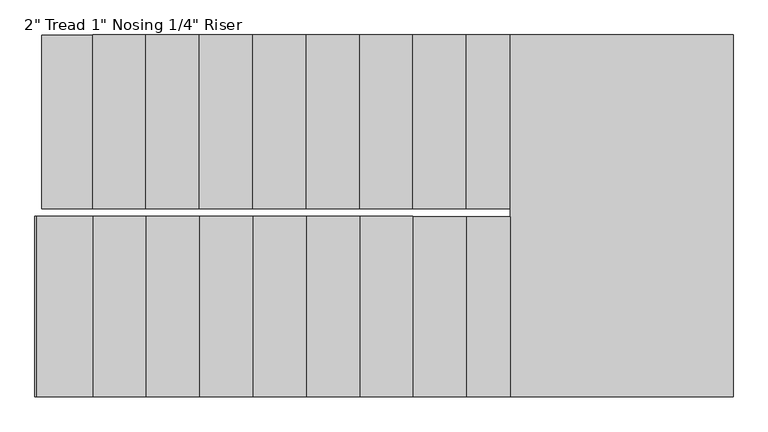
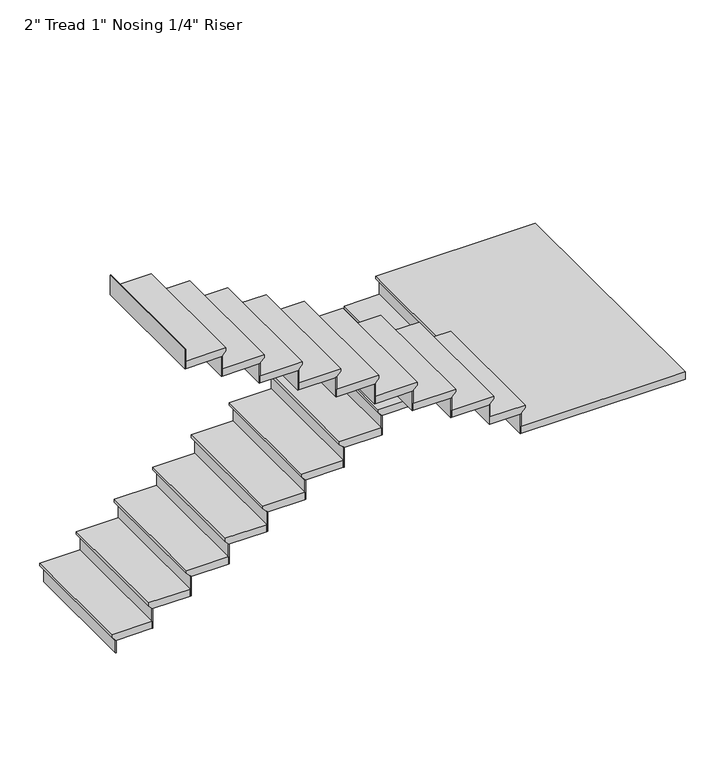
"""IFC4 building model written with IfcOpenShell, lengths in millimetres: stair flight geometry."""

from ifc_helpers import new_model, si_unit, origin, place, context, project, spatial, faceted_brep, source, transform, mapped, element, save


def stair_flight_3990532a(model_context):
    return source(origin(), model_context, "Body", "Brep", [
        faceted_brep([(1537.1941283, 180.9547293, 6214.11), (1537.1941283, 180.9547293, 6233.16), (1537.1941283, 1006.4547293, 6233.16), (1537.1941283, 1006.4547293, 6214.11), (1562.5941283, 180.9547293, 6188.71), (1562.5941283, 1006.4547293, 6188.71), (1804.8381368, 180.9547293, 6233.16), (1804.8381368, 1006.4547293, 6233.16), (1562.5941283, 1006.4547293, 6182.36), (1804.8381368, 1006.4547293, 6182.36), (1804.8381368, 180.9547293, 6182.36), (1562.5941283, 180.9547293, 6182.36)], [[[0, 1, 2, 3]], [[4, 0, 3, 5]], [[2, 1, 6, 7]], [[8, 9, 10, 11]], [[2, 7, 9, 8, 5, 3]], [[8, 11, 4, 5]], [[6, 1, 0, 4, 11, 10]], [[7, 6, 10, 9]]]),
        faceted_brep([(1562.5941283, 180.9547293, 6182.36), (1562.5941283, 180.9547293, 6096.0), (1568.9441283, 180.9547293, 6096.0), (1568.9441283, 180.9547293, 6182.36), (1562.5941283, 1006.4547293, 6182.36), (1568.9441283, 1006.4547293, 6182.36), (1568.9441283, 1006.4547293, 6096.0), (1562.5941283, 1006.4547293, 6096.0)], [[[0, 1, 2, 3]], [[4, 5, 6, 7]], [[1, 0, 4, 7]], [[2, 1, 7, 6]], [[3, 2, 6, 5]], [[0, 3, 5, 4]]]),
        faceted_brep([(1804.8381368, 180.9547293, 6319.52), (1804.8381368, 180.9547293, 6182.36), (1811.1881368, 180.9547293, 6182.36), (1811.1881368, 180.9547293, 6319.52), (1804.8381368, 1006.4547293, 6319.52), (1811.1881368, 1006.4547293, 6319.52), (1811.1881368, 1006.4547293, 6182.36), (1804.8381368, 1006.4547293, 6182.36)], [[[0, 1, 2, 3]], [[4, 5, 6, 7]], [[1, 0, 4, 7]], [[2, 1, 7, 6]], [[3, 2, 6, 5]], [[0, 3, 5, 4]]]),
        faceted_brep([(1779.4381368, 1006.4547293, 6370.32), (1779.4381368, 180.9547293, 6370.32), (2058.8381368, 180.9547293, 6370.32), (2058.8381368, 1006.4547293, 6370.32), (1804.8381368, 1006.4547293, 6319.52), (2058.8381368, 1006.4547293, 6319.52), (2058.8381368, 180.9547293, 6319.52), (1804.8381368, 180.9547293, 6319.52), (1804.8381368, 1006.4547293, 6325.87), (1779.4381368, 1006.4547293, 6351.27), (1804.8381368, 180.9547293, 6325.87), (1779.4381368, 180.9547293, 6351.27)], [[[0, 1, 2, 3]], [[4, 5, 6, 7]], [[0, 3, 5, 4, 8, 9]], [[4, 7, 10, 8]], [[2, 1, 11, 10, 7, 6]], [[3, 2, 6, 5]], [[11, 1, 0, 9]], [[10, 11, 9, 8]]]),
        faceted_brep([(2058.8381368, 180.9547293, 6456.68), (2058.8381368, 180.9547293, 6319.52), (2065.1881368, 180.9547293, 6319.52), (2065.1881368, 180.9547293, 6456.68), (2058.8381368, 1006.4547293, 6456.68), (2065.1881368, 1006.4547293, 6456.68), (2065.1881368, 1006.4547293, 6319.52), (2058.8381368, 1006.4547293, 6319.52)], [[[0, 1, 2, 3]], [[4, 5, 6, 7]], [[1, 0, 4, 7]], [[2, 1, 7, 6]], [[3, 2, 6, 5]], [[0, 3, 5, 4]]]),
        faceted_brep([(2033.4381368, 1006.4547293, 6507.48), (2033.4381368, 180.9547293, 6507.48), (2312.8381368, 180.9547293, 6507.48), (2312.8381368, 1006.4547293, 6507.48), (2058.8381368, 1006.4547293, 6456.68), (2312.8381368, 1006.4547293, 6456.68), (2312.8381368, 180.9547293, 6456.68), (2058.8381368, 180.9547293, 6456.68), (2058.8381368, 1006.4547293, 6463.03), (2033.4381368, 1006.4547293, 6488.43), (2058.8381368, 180.9547293, 6463.03), (2033.4381368, 180.9547293, 6488.43)], [[[0, 1, 2, 3]], [[4, 5, 6, 7]], [[0, 3, 5, 4, 8, 9]], [[4, 7, 10, 8]], [[2, 1, 11, 10, 7, 6]], [[3, 2, 6, 5]], [[11, 1, 0, 9]], [[10, 11, 9, 8]]]),
        faceted_brep([(2312.8381368, 180.9547293, 6593.84), (2312.8381368, 180.9547293, 6456.68), (2319.1881368, 180.9547293, 6456.68), (2319.1881368, 180.9547293, 6593.84), (2312.8381368, 1006.4547293, 6593.84), (2319.1881368, 1006.4547293, 6593.84), (2319.1881368, 1006.4547293, 6456.68), (2312.8381368, 1006.4547293, 6456.68)], [[[0, 1, 2, 3]], [[4, 5, 6, 7]], [[1, 0, 4, 7]], [[2, 1, 7, 6]], [[3, 2, 6, 5]], [[0, 3, 5, 4]]]),
        faceted_brep([(2287.4381368, 1006.4547293, 6644.64), (2287.4381368, 180.9547293, 6644.64), (2566.8381368, 180.9547293, 6644.64), (2566.8381368, 1006.4547293, 6644.64), (2312.8381368, 1006.4547293, 6593.84), (2566.8381368, 1006.4547293, 6593.84), (2566.8381368, 180.9547293, 6593.84), (2312.8381368, 180.9547293, 6593.84), (2312.8381368, 1006.4547293, 6600.19), (2287.4381368, 1006.4547293, 6625.59), (2312.8381368, 180.9547293, 6600.19), (2287.4381368, 180.9547293, 6625.59)], [[[0, 1, 2, 3]], [[4, 5, 6, 7]], [[0, 3, 5, 4, 8, 9]], [[4, 7, 10, 8]], [[2, 1, 11, 10, 7, 6]], [[3, 2, 6, 5]], [[11, 1, 0, 9]], [[10, 11, 9, 8]]]),
        faceted_brep([(2566.8381368, 180.9547293, 6731.0), (2566.8381368, 180.9547293, 6593.84), (2573.1881368, 180.9547293, 6593.84), (2573.1881368, 180.9547293, 6731.0), (2566.8381368, 1006.4547293, 6731.0), (2573.1881368, 1006.4547293, 6731.0), (2573.1881368, 1006.4547293, 6593.84), (2566.8381368, 1006.4547293, 6593.84)], [[[0, 1, 2, 3]], [[4, 5, 6, 7]], [[1, 0, 4, 7]], [[2, 1, 7, 6]], [[3, 2, 6, 5]], [[0, 3, 5, 4]]]),
        faceted_brep([(2541.4381368, 1006.4547293, 6781.8), (2541.4381368, 180.9547293, 6781.8), (2820.8381368, 180.9547293, 6781.8), (2820.8381368, 1006.4547293, 6781.8), (2566.8381368, 1006.4547293, 6731.0), (2820.8381368, 1006.4547293, 6731.0), (2820.8381368, 180.9547293, 6731.0), (2566.8381368, 180.9547293, 6731.0), (2566.8381368, 1006.4547293, 6737.35), (2541.4381368, 1006.4547293, 6762.75), (2566.8381368, 180.9547293, 6737.35), (2541.4381368, 180.9547293, 6762.75)], [[[0, 1, 2, 3]], [[4, 5, 6, 7]], [[0, 3, 5, 4, 8, 9]], [[4, 7, 10, 8]], [[2, 1, 11, 10, 7, 6]], [[3, 2, 6, 5]], [[11, 1, 0, 9]], [[10, 11, 9, 8]]]),
        faceted_brep([(2820.8381368, 180.9547293, 6868.16), (2820.8381368, 180.9547293, 6731.0), (2827.1881368, 180.9547293, 6731.0), (2827.1881368, 180.9547293, 6868.16), (2820.8381368, 1006.4547293, 6868.16), (2827.1881368, 1006.4547293, 6868.16), (2827.1881368, 1006.4547293, 6731.0), (2820.8381368, 1006.4547293, 6731.0)], [[[0, 1, 2, 3]], [[4, 5, 6, 7]], [[1, 0, 4, 7]], [[2, 1, 7, 6]], [[3, 2, 6, 5]], [[0, 3, 5, 4]]]),
        faceted_brep([(2795.4381368, 1006.4547293, 6918.96), (2795.4381368, 180.9547293, 6918.96), (3074.8381368, 180.9547293, 6918.96), (3074.8381368, 1006.4547293, 6918.96), (2820.8381368, 1006.4547293, 6868.16), (3074.8381368, 1006.4547293, 6868.16), (3074.8381368, 180.9547293, 6868.16), (2820.8381368, 180.9547293, 6868.16), (2820.8381368, 1006.4547293, 6874.51), (2795.4381368, 1006.4547293, 6899.91), (2820.8381368, 180.9547293, 6874.51), (2795.4381368, 180.9547293, 6899.91)], [[[0, 1, 2, 3]], [[4, 5, 6, 7]], [[0, 3, 5, 4, 8, 9]], [[4, 7, 10, 8]], [[2, 1, 11, 10, 7, 6]], [[3, 2, 6, 5]], [[11, 1, 0, 9]], [[10, 11, 9, 8]]]),
        faceted_brep([(3074.8381368, 180.9547293, 7005.32), (3074.8381368, 180.9547293, 6868.16), (3081.1881368, 180.9547293, 6868.16), (3081.1881368, 180.9547293, 7005.32), (3074.8381368, 1006.4547293, 7005.32), (3081.1881368, 1006.4547293, 7005.32), (3081.1881368, 1006.4547293, 6868.16), (3074.8381368, 1006.4547293, 6868.16)], [[[0, 1, 2, 3]], [[4, 5, 6, 7]], [[1, 0, 4, 7]], [[2, 1, 7, 6]], [[3, 2, 6, 5]], [[0, 3, 5, 4]]]),
        faceted_brep([(3049.4381368, 1006.4547293, 7056.12), (3049.4381368, 180.9547293, 7056.12), (3328.8381368, 180.9547293, 7056.12), (3328.8381368, 1006.4547293, 7056.12), (3074.8381368, 1006.4547293, 7005.32), (3328.8381368, 1006.4547293, 7005.32), (3328.8381368, 180.9547293, 7005.32), (3074.8381368, 180.9547293, 7005.32), (3074.8381368, 1006.4547293, 7011.67), (3049.4381368, 1006.4547293, 7037.07), (3074.8381368, 180.9547293, 7011.67), (3049.4381368, 180.9547293, 7037.07)], [[[0, 1, 2, 3]], [[4, 5, 6, 7]], [[0, 3, 5, 4, 8, 9]], [[4, 7, 10, 8]], [[2, 1, 11, 10, 7, 6]], [[3, 2, 6, 5]], [[11, 1, 0, 9]], [[10, 11, 9, 8]]]),
        faceted_brep([(3328.8381368, 180.9547293, 7142.48), (3328.8381368, 180.9547293, 7005.32), (3335.1881368, 180.9547293, 7005.32), (3335.1881368, 180.9547293, 7142.48), (3328.8381368, 1006.4547293, 7142.48), (3335.1881368, 1006.4547293, 7142.48), (3335.1881368, 1006.4547293, 7005.32), (3328.8381368, 1006.4547293, 7005.32)], [[[0, 1, 2, 3]], [[4, 5, 6, 7]], [[1, 0, 4, 7]], [[2, 1, 7, 6]], [[3, 2, 6, 5]], [[0, 3, 5, 4]]]),
        faceted_brep([(3303.4381368, 1006.4547293, 7193.28), (3303.4381368, 180.9547293, 7193.28), (3582.8381368, 180.9547293, 7193.28), (3582.8381368, 1006.4547293, 7193.28), (3328.8381368, 1006.4547293, 7142.48), (3582.8381368, 1006.4547293, 7142.48), (3582.8381368, 180.9547293, 7142.48), (3328.8381368, 180.9547293, 7142.48), (3328.8381368, 1006.4547293, 7148.83), (3303.4381368, 1006.4547293, 7174.23), (3328.8381368, 180.9547293, 7148.83), (3303.4381368, 180.9547293, 7174.23)], [[[0, 1, 2, 3]], [[4, 5, 6, 7]], [[0, 3, 5, 4, 8, 9]], [[4, 7, 10, 8]], [[2, 1, 11, 10, 7, 6]], [[3, 2, 6, 5]], [[11, 1, 0, 9]], [[10, 11, 9, 8]]]),
        faceted_brep([(3582.8381368, 180.9547293, 7279.64), (3582.8381368, 180.9547293, 7142.48), (3589.1881368, 180.9547293, 7142.48), (3589.1881368, 180.9547293, 7279.64), (3582.8381368, 1006.4547293, 7279.64), (3589.1881368, 1006.4547293, 7279.64), (3589.1881368, 1006.4547293, 7142.48), (3582.8381368, 1006.4547293, 7142.48)], [[[0, 1, 2, 3]], [[4, 5, 6, 7]], [[1, 0, 4, 7]], [[2, 1, 7, 6]], [[3, 2, 6, 5]], [[0, 3, 5, 4]]]),
        faceted_brep([(3557.4381368, 1006.4547293, 7330.44), (3557.4381368, 180.9547293, 7330.44), (3791.2648053, 180.9547293, 7330.44), (3791.2648053, 1006.4547293, 7330.44), (3582.8381368, 1006.4547293, 7279.64), (3791.2648053, 1006.4547293, 7279.64), (3791.2648053, 180.9547293, 7279.64), (3582.8381368, 180.9547293, 7279.64), (3582.8381368, 1006.4547293, 7285.99), (3557.4381368, 1006.4547293, 7311.39), (3582.8381368, 180.9547293, 7285.99), (3557.4381368, 180.9547293, 7311.39)], [[[0, 1, 2, 3]], [[4, 5, 6, 7]], [[0, 3, 5, 4, 8, 9]], [[4, 7, 10, 8]], [[2, 1, 11, 10, 7, 6]], [[3, 2, 6, 5]], [[11, 1, 0, 9]], [[10, 11, 9, 8]]]),
        faceted_brep([(3791.2648053, 180.9547293, 7416.8), (3791.2648053, 180.9547293, 7279.64), (3797.6148053, 180.9547293, 7279.64), (3797.6148053, 180.9547293, 7416.8), (3791.2648053, 1006.4547293, 7416.8), (3797.6148053, 1006.4547293, 7416.8), (3797.6148053, 1006.4547293, 7279.64), (3791.2648053, 1006.4547293, 7279.64)], [[[0, 1, 2, 3]], [[4, 5, 6, 7]], [[1, 0, 4, 7]], [[2, 1, 7, 6]], [[3, 2, 6, 5]], [[0, 3, 5, 4]]]),
        faceted_brep([(3740.4648053, -714.2964201, 7467.6), (4826.4941283, -714.2964201, 7467.6), (4826.4941283, 1006.4547293, 7467.6), (3765.8648053, 1006.4547293, 7467.6), (3765.8648053, 142.8547293, 7467.6), (3740.4648053, 142.8547293, 7467.6), (4826.4941283, -714.2964201, 7416.8), (3740.4648053, -714.2964201, 7416.8), (3740.4648053, 142.8547293, 7416.8), (3765.8648053, 142.8547293, 7416.8), (3765.8648053, 180.9547293, 7416.8), (3791.2648053, 180.9547293, 7416.8), (3791.2648053, 1006.4547293, 7416.8), (4826.4941283, 1006.4547293, 7416.8), (3791.2648053, 1006.4547293, 7423.15), (3765.8648053, 1006.4547293, 7448.55), (3791.2648053, 180.9547293, 7423.15), (3765.8648053, 180.9547293, 7448.55)], [[[0, 1, 2, 3, 4, 5]], [[6, 7, 8, 9, 10, 11, 12, 13]], [[1, 0, 7, 6]], [[2, 1, 6, 13]], [[3, 2, 13, 12, 14, 15]], [[12, 11, 16, 14]], [[11, 10, 17, 16]], [[4, 3, 15, 17, 10, 9]], [[5, 4, 9, 8]], [[0, 5, 8, 7]], [[15, 14, 16, 17]]]),
        faceted_brep([(3740.4648053, 142.8547293, 7553.96), (3740.4648053, 142.8547293, 7416.8), (3734.1148053, 142.8547293, 7416.8), (3734.1148053, 142.8547293, 7553.96), (3740.4648053, -714.2964201, 7553.96), (3734.1148053, -714.2964201, 7553.96), (3734.1148053, -714.2964201, 7416.8), (3740.4648053, -714.2964201, 7416.8)], [[[0, 1, 2, 3]], [[4, 5, 6, 7]], [[1, 0, 4, 7]], [[2, 1, 7, 6]], [[3, 2, 6, 5]], [[0, 3, 5, 4]]]),
        faceted_brep([(3765.8648053, -714.2964201, 7604.76), (3765.8648053, 142.8547293, 7604.76), (3532.0381368, 142.8547293, 7604.76), (3532.0381368, -714.2964201, 7604.76), (3740.4648053, -714.2964201, 7553.96), (3532.0381368, -714.2964201, 7553.96), (3532.0381368, 142.8547293, 7553.96), (3740.4648053, 142.8547293, 7553.96), (3740.4648053, -714.2964201, 7560.31), (3765.8648053, -714.2964201, 7585.71), (3740.4648053, 142.8547293, 7560.31), (3765.8648053, 142.8547293, 7585.71)], [[[0, 1, 2, 3]], [[4, 5, 6, 7]], [[0, 3, 5, 4, 8, 9]], [[4, 7, 10, 8]], [[2, 1, 11, 10, 7, 6]], [[3, 2, 6, 5]], [[11, 1, 0, 9]], [[10, 11, 9, 8]]]),
        faceted_brep([(3532.0381368, 142.8547293, 7691.12), (3532.0381368, 142.8547293, 7553.96), (3525.6881368, 142.8547293, 7553.96), (3525.6881368, 142.8547293, 7691.12), (3532.0381368, -714.2964201, 7691.12), (3525.6881368, -714.2964201, 7691.12), (3525.6881368, -714.2964201, 7553.96), (3532.0381368, -714.2964201, 7553.96)], [[[0, 1, 2, 3]], [[4, 5, 6, 7]], [[1, 0, 4, 7]], [[2, 1, 7, 6]], [[3, 2, 6, 5]], [[0, 3, 5, 4]]]),
        faceted_brep([(3557.4381368, -714.2964201, 7741.92), (3557.4381368, 142.8547293, 7741.92), (3278.0381368, 142.8547293, 7741.92), (3278.0381368, -714.2964201, 7741.92), (3532.0381368, -714.2964201, 7691.12), (3278.0381368, -714.2964201, 7691.12), (3278.0381368, 142.8547293, 7691.12), (3532.0381368, 142.8547293, 7691.12), (3532.0381368, -714.2964201, 7697.47), (3557.4381368, -714.2964201, 7722.87), (3532.0381368, 142.8547293, 7697.47), (3557.4381368, 142.8547293, 7722.87)], [[[0, 1, 2, 3]], [[4, 5, 6, 7]], [[0, 3, 5, 4, 8, 9]], [[4, 7, 10, 8]], [[2, 1, 11, 10, 7, 6]], [[3, 2, 6, 5]], [[11, 1, 0, 9]], [[10, 11, 9, 8]]]),
        faceted_brep([(3278.0381368, 142.8547293, 7828.28), (3278.0381368, 142.8547293, 7691.12), (3271.6881368, 142.8547293, 7691.12), (3271.6881368, 142.8547293, 7828.28), (3278.0381368, -714.2964201, 7828.28), (3271.6881368, -714.2964201, 7828.28), (3271.6881368, -714.2964201, 7691.12), (3278.0381368, -714.2964201, 7691.12)], [[[0, 1, 2, 3]], [[4, 5, 6, 7]], [[1, 0, 4, 7]], [[2, 1, 7, 6]], [[3, 2, 6, 5]], [[0, 3, 5, 4]]]),
        faceted_brep([(3303.4381368, -714.2964201, 7879.08), (3303.4381368, 142.8547293, 7879.08), (3024.0381368, 142.8547293, 7879.08), (3024.0381368, -714.2964201, 7879.08), (3278.0381368, -714.2964201, 7828.28), (3024.0381368, -714.2964201, 7828.28), (3024.0381368, 142.8547293, 7828.28), (3278.0381368, 142.8547293, 7828.28), (3278.0381368, -714.2964201, 7834.63), (3303.4381368, -714.2964201, 7860.03), (3278.0381368, 142.8547293, 7834.63), (3303.4381368, 142.8547293, 7860.03)], [[[0, 1, 2, 3]], [[4, 5, 6, 7]], [[0, 3, 5, 4, 8, 9]], [[4, 7, 10, 8]], [[2, 1, 11, 10, 7, 6]], [[3, 2, 6, 5]], [[11, 1, 0, 9]], [[10, 11, 9, 8]]]),
        faceted_brep([(3024.0381368, 142.8547293, 7965.44), (3024.0381368, 142.8547293, 7828.28), (3017.6881368, 142.8547293, 7828.28), (3017.6881368, 142.8547293, 7965.44), (3024.0381368, -714.2964201, 7965.44), (3017.6881368, -714.2964201, 7965.44), (3017.6881368, -714.2964201, 7828.28), (3024.0381368, -714.2964201, 7828.28)], [[[0, 1, 2, 3]], [[4, 5, 6, 7]], [[1, 0, 4, 7]], [[2, 1, 7, 6]], [[3, 2, 6, 5]], [[0, 3, 5, 4]]]),
        faceted_brep([(3049.4381368, -714.2964201, 8016.24), (3049.4381368, 142.8547293, 8016.24), (2770.0381368, 142.8547293, 8016.24), (2770.0381368, -714.2964201, 8016.24), (3024.0381368, -714.2964201, 7965.44), (2770.0381368, -714.2964201, 7965.44), (2770.0381368, 142.8547293, 7965.44), (3024.0381368, 142.8547293, 7965.44), (3024.0381368, -714.2964201, 7971.79), (3049.4381368, -714.2964201, 7997.19), (3024.0381368, 142.8547293, 7971.79), (3049.4381368, 142.8547293, 7997.19)], [[[0, 1, 2, 3]], [[4, 5, 6, 7]], [[0, 3, 5, 4, 8, 9]], [[4, 7, 10, 8]], [[2, 1, 11, 10, 7, 6]], [[3, 2, 6, 5]], [[11, 1, 0, 9]], [[10, 11, 9, 8]]]),
        faceted_brep([(2770.0381368, 142.8547293, 8102.6), (2770.0381368, 142.8547293, 7965.44), (2763.6881368, 142.8547293, 7965.44), (2763.6881368, 142.8547293, 8102.6), (2770.0381368, -714.2964201, 8102.6), (2763.6881368, -714.2964201, 8102.6), (2763.6881368, -714.2964201, 7965.44), (2770.0381368, -714.2964201, 7965.44)], [[[0, 1, 2, 3]], [[4, 5, 6, 7]], [[1, 0, 4, 7]], [[2, 1, 7, 6]], [[3, 2, 6, 5]], [[0, 3, 5, 4]]]),
        faceted_brep([(2795.4381368, -714.2964201, 8153.4), (2795.4381368, 142.8547293, 8153.4), (2516.0381368, 142.8547293, 8153.4), (2516.0381368, -714.2964201, 8153.4), (2770.0381368, -714.2964201, 8102.6), (2516.0381368, -714.2964201, 8102.6), (2516.0381368, 142.8547293, 8102.6), (2770.0381368, 142.8547293, 8102.6), (2770.0381368, -714.2964201, 8108.95), (2795.4381368, -714.2964201, 8134.35), (2770.0381368, 142.8547293, 8108.95), (2795.4381368, 142.8547293, 8134.35)], [[[0, 1, 2, 3]], [[4, 5, 6, 7]], [[0, 3, 5, 4, 8, 9]], [[4, 7, 10, 8]], [[2, 1, 11, 10, 7, 6]], [[3, 2, 6, 5]], [[11, 1, 0, 9]], [[10, 11, 9, 8]]]),
        faceted_brep([(2516.0381368, 142.8547293, 8239.76), (2516.0381368, 142.8547293, 8102.6), (2509.6881368, 142.8547293, 8102.6), (2509.6881368, 142.8547293, 8239.76), (2516.0381368, -714.2964201, 8239.76), (2509.6881368, -714.2964201, 8239.76), (2509.6881368, -714.2964201, 8102.6), (2516.0381368, -714.2964201, 8102.6)], [[[0, 1, 2, 3]], [[4, 5, 6, 7]], [[1, 0, 4, 7]], [[2, 1, 7, 6]], [[3, 2, 6, 5]], [[0, 3, 5, 4]]]),
        faceted_brep([(2541.4381368, -714.2964201, 8290.56), (2541.4381368, 142.8547293, 8290.56), (2262.0381368, 142.8547293, 8290.56), (2262.0381368, -714.2964201, 8290.56), (2516.0381368, -714.2964201, 8239.76), (2262.0381368, -714.2964201, 8239.76), (2262.0381368, 142.8547293, 8239.76), (2516.0381368, 142.8547293, 8239.76), (2516.0381368, -714.2964201, 8246.11), (2541.4381368, -714.2964201, 8271.51), (2516.0381368, 142.8547293, 8246.11), (2541.4381368, 142.8547293, 8271.51)], [[[0, 1, 2, 3]], [[4, 5, 6, 7]], [[0, 3, 5, 4, 8, 9]], [[4, 7, 10, 8]], [[2, 1, 11, 10, 7, 6]], [[3, 2, 6, 5]], [[11, 1, 0, 9]], [[10, 11, 9, 8]]]),
        faceted_brep([(2262.0381368, 142.8547293, 8376.92), (2262.0381368, 142.8547293, 8239.76), (2255.6881368, 142.8547293, 8239.76), (2255.6881368, 142.8547293, 8376.92), (2262.0381368, -714.2964201, 8376.92), (2255.6881368, -714.2964201, 8376.92), (2255.6881368, -714.2964201, 8239.76), (2262.0381368, -714.2964201, 8239.76)], [[[0, 1, 2, 3]], [[4, 5, 6, 7]], [[1, 0, 4, 7]], [[2, 1, 7, 6]], [[3, 2, 6, 5]], [[0, 3, 5, 4]]]),
        faceted_brep([(2287.4381368, -714.2964201, 8427.72), (2287.4381368, 142.8547293, 8427.72), (2008.0381368, 142.8547293, 8427.72), (2008.0381368, -714.2964201, 8427.72), (2262.0381368, -714.2964201, 8376.92), (2008.0381368, -714.2964201, 8376.92), (2008.0381368, 142.8547293, 8376.92), (2262.0381368, 142.8547293, 8376.92), (2262.0381368, -714.2964201, 8383.27), (2287.4381368, -714.2964201, 8408.67), (2262.0381368, 142.8547293, 8383.27), (2287.4381368, 142.8547293, 8408.67)], [[[0, 1, 2, 3]], [[4, 5, 6, 7]], [[0, 3, 5, 4, 8, 9]], [[4, 7, 10, 8]], [[2, 1, 11, 10, 7, 6]], [[3, 2, 6, 5]], [[11, 1, 0, 9]], [[10, 11, 9, 8]]]),
        faceted_brep([(2008.0381368, 142.8547293, 8514.08), (2008.0381368, 142.8547293, 8376.92), (2001.6881368, 142.8547293, 8376.92), (2001.6881368, 142.8547293, 8514.08), (2008.0381368, -714.2964201, 8514.08), (2001.6881368, -714.2964201, 8514.08), (2001.6881368, -714.2964201, 8376.92), (2008.0381368, -714.2964201, 8376.92)], [[[0, 1, 2, 3]], [[4, 5, 6, 7]], [[1, 0, 4, 7]], [[2, 1, 7, 6]], [[3, 2, 6, 5]], [[0, 3, 5, 4]]]),
        faceted_brep([(2033.4381368, -714.2964201, 8564.88), (2033.4381368, 142.8547293, 8564.88), (1754.0381368, 142.8547293, 8564.88), (1754.0381368, -714.2964201, 8564.88), (2008.0381368, -714.2964201, 8514.08), (1754.0381368, -714.2964201, 8514.08), (1754.0381368, 142.8547293, 8514.08), (2008.0381368, 142.8547293, 8514.08), (2008.0381368, -714.2964201, 8520.43), (2033.4381368, -714.2964201, 8545.83), (2008.0381368, 142.8547293, 8520.43), (2033.4381368, 142.8547293, 8545.83)], [[[0, 1, 2, 3]], [[4, 5, 6, 7]], [[0, 3, 5, 4, 8, 9]], [[4, 7, 10, 8]], [[2, 1, 11, 10, 7, 6]], [[3, 2, 6, 5]], [[11, 1, 0, 9]], [[10, 11, 9, 8]]]),
        faceted_brep([(1754.0381368, 142.8547293, 8651.24), (1754.0381368, 142.8547293, 8514.08), (1747.6881368, 142.8547293, 8514.08), (1747.6881368, 142.8547293, 8651.24), (1754.0381368, -714.2964201, 8651.24), (1747.6881368, -714.2964201, 8651.24), (1747.6881368, -714.2964201, 8514.08), (1754.0381368, -714.2964201, 8514.08)], [[[0, 1, 2, 3]], [[4, 5, 6, 7]], [[1, 0, 4, 7]], [[2, 1, 7, 6]], [[3, 2, 6, 5]], [[0, 3, 5, 4]]]),
        faceted_brep([(1511.7941283, 142.8547293, 8788.4), (1511.7941283, 142.8547293, 8651.24), (1505.4441283, 142.8547293, 8651.24), (1505.4441283, 142.8547293, 8788.4), (1511.7941283, -714.2964201, 8788.4), (1505.4441283, -714.2964201, 8788.4), (1505.4441283, -714.2964201, 8651.24), (1511.7941283, -714.2964201, 8651.24)], [[[0, 1, 2, 3]], [[4, 5, 6, 7]], [[1, 0, 4, 7]], [[2, 1, 7, 6]], [[3, 2, 6, 5]], [[0, 3, 5, 4]]]),
        faceted_brep([(1779.4381368, -714.2964201, 8702.04), (1779.4381368, 142.8547293, 8702.04), (1511.7941283, 142.8547293, 8702.04), (1511.7941283, -714.2964201, 8702.04), (1754.0381368, -714.2964201, 8651.24), (1511.7941283, -714.2964201, 8651.24), (1511.7941283, 142.8547293, 8651.24), (1754.0381368, 142.8547293, 8651.24), (1754.0381368, -714.2964201, 8657.59), (1779.4381368, -714.2964201, 8682.99), (1754.0381368, 142.8547293, 8657.59), (1779.4381368, 142.8547293, 8682.99)], [[[0, 1, 2, 3]], [[4, 5, 6, 7]], [[0, 3, 5, 4, 8, 9]], [[4, 7, 10, 8]], [[2, 1, 11, 10, 7, 6]], [[3, 2, 6, 5]], [[11, 1, 0, 9]], [[10, 11, 9, 8]]]),
    ])


if __name__ == "__main__":
    model = new_model("IFC4")
    model_context = context("Model", 3, world=origin())
    ifc_project = project(units=[si_unit("LENGTHUNIT", "METRE", prefix="MILLI")], contexts=[model_context])
    site = spatial("IfcSite", under=ifc_project)
    building = spatial("IfcBuilding", under=site)
    placement = place(None, origin())
    stair_flight_shape = stair_flight_3990532a(model_context)
    element("IfcStairFlight", 1, ObjectType="2\" Tread 1\" Nosing 1/4\" Riser", at=placement, inside=building, context=model_context, shape_type="MappedRepresentation", body=[
        mapped(stair_flight_shape, transform((0.0, 0.0, 0.0), x_axis=(1.0, 0.0, 0.0), y_axis=(0.0, 1.0, 0.0), z_axis=(0.0, 0.0, 1.0))),
    ])
    save(model, "model.ifc")
